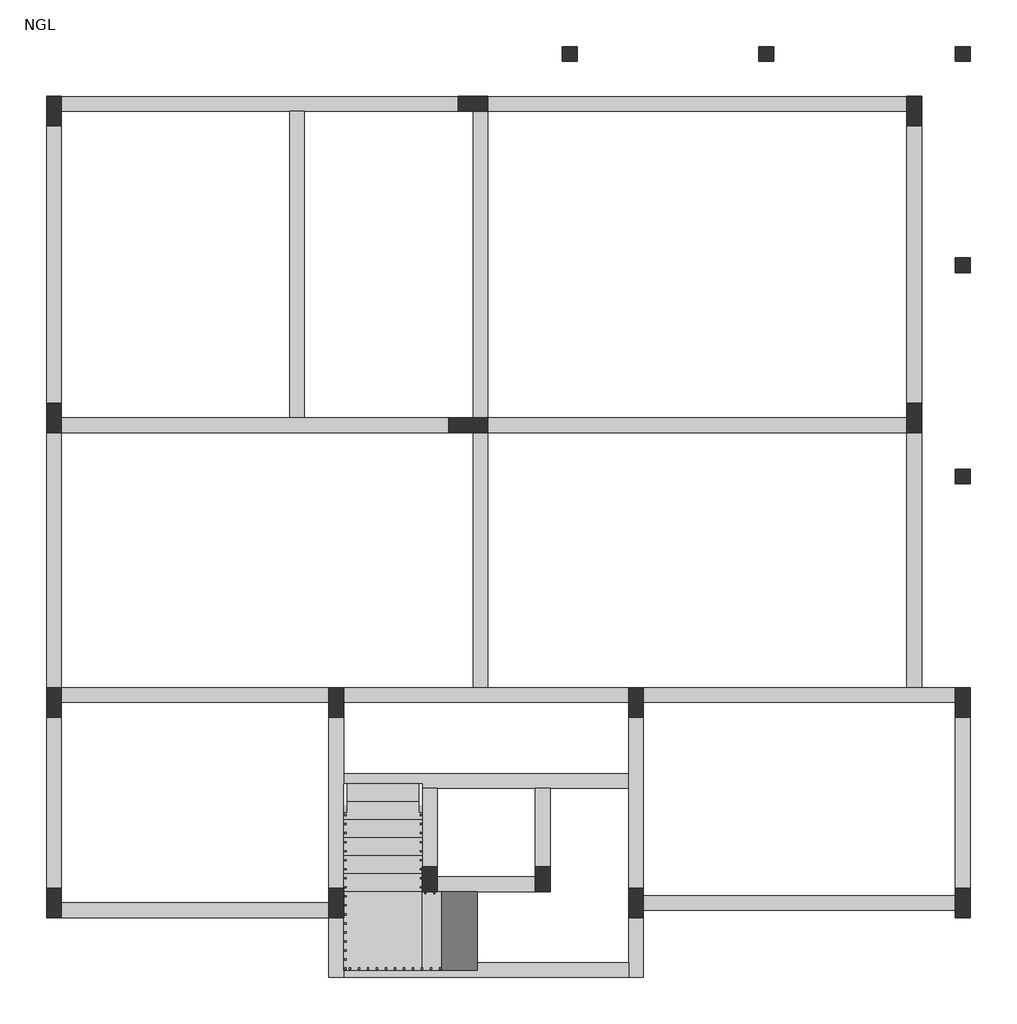
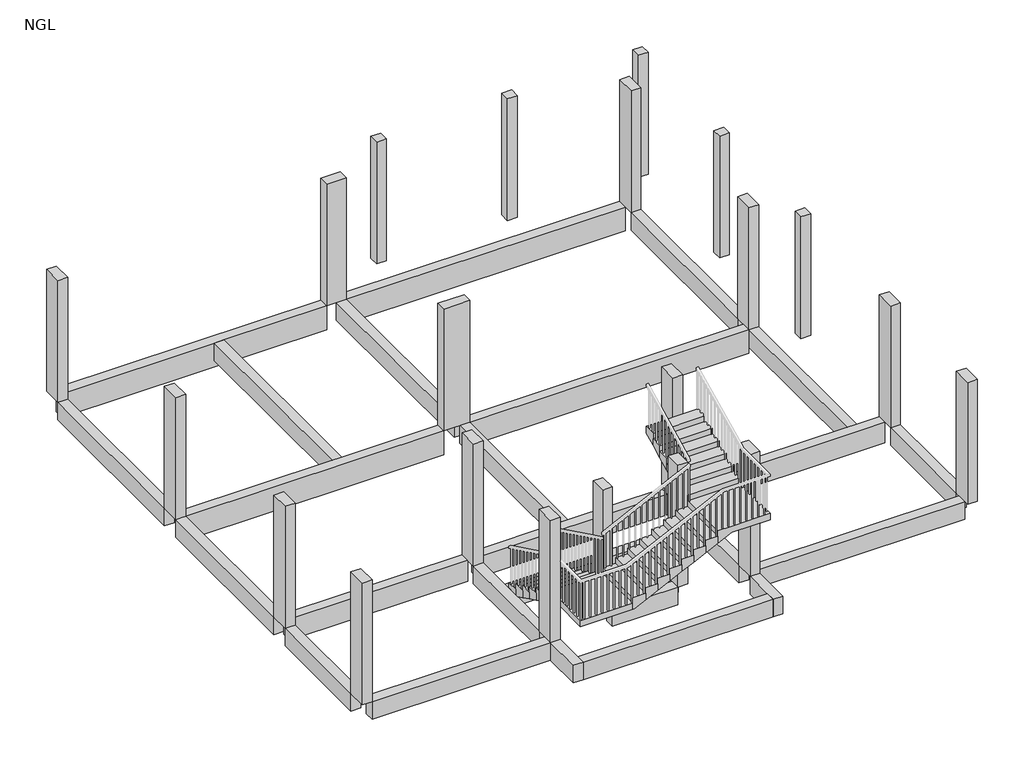
# One storey, part 1 of 2: 27 beams, 21 columns, 1 stair flight.
"""IFC4 building model written with IfcOpenShell, lengths in millimetres."""

from ifc_helpers import new_model, si_unit, frame, origin, origin_with_axes, place, context, project, spatial, polyline, outline, extrude, faceted_brep, transform, mapped, element, save
from components import concrete_rectangular_column_c_80bd43f1

model = new_model("IFC4")

# Units and contexts
model_context = context("Model", 3, world=origin())
ifc_project = project(units=[si_unit("LENGTHUNIT", "METRE", prefix="MILLI")], contexts=[model_context])

# Site, building, storey
site = spatial("IfcSite", under=ifc_project)
building = spatial("IfcBuilding", under=site)
storey = spatial("IfcBuildingStorey", under=building, Name="NGL", Elevation=0.0)

# Beams
placement = place(None, origin())
element("IfcBeam", 1, ObjectType="Concrete - Rectangular Beam : B1", at=placement, inside=storey, context=model_context, shape_type="Brep", body=[
    faceted_brep([(5662813.1113073, -3585265.1224803, 0.0), (5662813.1113073, -3585493.7224803, 0.0), (5666356.4266467, -3585493.7224803, 0.0), (5666585.0266467, -3585493.7224803, 0.0), (5668972.6206949, -3585493.7224803, 0.0), (5668972.6206949, -3585265.1224803, 0.0), (5662813.1113073, -3585493.7224803, -584.2), (5668972.6206949, -3585493.7224803, -584.2), (5662813.1113073, -3585265.1224803, -584.2), (5668972.6206949, -3585265.1224803, -584.2)], [[[0, 1, 2, 3, 4, 5]], [[1, 6, 7, 4, 3, 2]], [[6, 8, 9, 7]], [[8, 0, 5, 9]], [[1, 0, 8, 6]], [[5, 4, 7, 9]]]),
])
element("IfcBeam", 2, ObjectType="Concrete - Rectangular Beam : B1", at=placement, inside=storey, context=model_context, shape_type="Brep", body=[
    faceted_brep([(5675932.2165246, -3585493.7224803, 0.0), (5675932.2165246, -3585265.1224803, 0.0), (5669429.8206949, -3585265.1224803, 0.0), (5669429.8297535, -3585493.7224803, 0.0), (5675932.2165246, -3585493.7224803, -584.2), (5669429.8206949, -3585493.7224803, -584.2), (5675932.2165246, -3585265.1224803, -584.2), (5669429.8206949, -3585265.1224803, -584.2)], [[[0, 1, 2, 3]], [[4, 0, 3, 5]], [[6, 4, 5, 7]], [[1, 6, 7, 2]], [[1, 0, 4, 6]], [[2, 7, 5, 3]]]),
])
element("IfcBeam", 3, ObjectType="Concrete - Rectangular Beam : B10", at=placement, inside=storey, context=model_context, shape_type="SweptSolid", body=[
    extrude(outline(polyline([(5670395.0165245, -3597217.2875145), (5670166.4165245, -3597217.2875145), (5670166.4165245, -3595998.1287586), (5670395.0165245, -3595998.1287586), (5670395.0165245, -3597217.2875145)])), frame((0.0, 0.0, -431.8), z_axis=(0.0, 0.0, 1.0), x_axis=(1.0, 0.0, 0.0)), (0.0, 0.0, 1.0), 431.8),
])
element("IfcBeam", 4, ObjectType="Concrete - Rectangular Beam : B10", at=placement, inside=storey, context=model_context, shape_type="SweptSolid", body=[
    extrude(outline(polyline([(5668642.4165246, -3597217.2875145), (5668413.8165246, -3597217.2875145), (5668413.8165246, -3595998.1287586), (5668642.4165246, -3595998.1287586), (5668642.4165246, -3597217.2875145)])), frame((0.0, 0.0, -431.8), z_axis=(0.0, 0.0, 1.0), x_axis=(1.0, 0.0, 0.0)), (0.0, 0.0, 1.0), 431.8),
])
element("IfcBeam", 5, ObjectType="Concrete - Rectangular Beam : B11", at=placement, inside=storey, context=model_context, shape_type="SweptSolid", body=[
    extrude(outline(polyline([(5669201.2297535, -3585493.7224803), (5669429.8297535, -3585493.7224803), (5669429.8297535, -3590249.6682909), (5669201.2297535, -3590249.6682909), (5669201.2297535, -3585493.7224803)])), frame((0.0, 0.0, -431.8), z_axis=(0.0, 0.0, 1.0), x_axis=(1.0, 0.0, 0.0)), (0.0, 0.0, 1.0), 431.8),
])
element("IfcBeam", 6, ObjectType="Concrete - Rectangular Beam : B11", at=placement, inside=storey, context=model_context, shape_type="SweptSolid", body=[
    extrude(outline(polyline([(5669201.2297535, -3590478.2682909), (5669429.8297535, -3590478.2682909), (5669429.8297535, -3594436.7630076), (5669201.2297535, -3594436.7630076), (5669201.2297535, -3590478.2682909)])), frame((0.0, 0.0, -431.8), z_axis=(0.0, 0.0, 1.0), x_axis=(1.0, 0.0, 0.0)), (0.0, 0.0, 1.0), 431.8),
])
element("IfcBeam", 7, ObjectType="Concrete - Rectangular Beam : B12", at=placement, inside=storey, context=model_context, shape_type="SweptSolid", body=[
    extrude(outline(polyline([(5675932.2165246, -3585722.3224803), (5676160.8165246, -3585722.3224803), (5676160.8165246, -3590021.0682909), (5675932.2165246, -3590021.0682909), (5675932.2165246, -3585722.3224803)])), frame((0.0, 0.0, -431.8), z_axis=(0.0, 0.0, 1.0), x_axis=(1.0, 0.0, 0.0)), (0.0, 0.0, 1.0), 431.8),
])
element("IfcBeam", 8, ObjectType="Concrete - Rectangular Beam : B12", at=placement, inside=storey, context=model_context, shape_type="SweptSolid", body=[
    extrude(outline(polyline([(5675932.2165246, -3590478.2682909), (5676160.8165246, -3590478.2682909), (5676160.8165246, -3594436.7630076), (5675932.2165246, -3594436.7630076), (5675932.2165246, -3590478.2682909)])), frame((0.0, 0.0, -431.8), z_axis=(0.0, 0.0, 1.0), x_axis=(1.0, 0.0, 0.0)), (0.0, 0.0, 1.0), 431.8),
])
element("IfcBeam", 9, ObjectType="Concrete - Rectangular Beam : B13", at=placement, inside=storey, context=model_context, shape_type="SweptSolid", body=[
    extrude(outline(polyline([(5676681.5650571, -3594893.8523052), (5676910.1650571, -3594893.8523052), (5676910.1650571, -3597545.8975754), (5676681.5650571, -3597545.8975754), (5676681.5650571, -3594893.8523052)])), frame((0.0, 0.0, -431.8), z_axis=(0.0, 0.0, 1.0), x_axis=(1.0, 0.0, 0.0)), (0.0, 0.0, 1.0), 431.8),
])
element("IfcBeam", 10, ObjectType="Concrete - Rectangular Beam : B2", at=placement, inside=storey, context=model_context, shape_type="Brep", body=[
    faceted_brep([(5668820.2206949, -3590478.2682909, 0.0), (5668820.2206949, -3590249.6682909, 0.0), (5666585.0266467, -3590249.6682909, 0.0), (5666356.4266467, -3590249.6682909, 0.0), (5662813.1650571, -3590249.6682909, 0.0), (5662813.1650571, -3590478.2682909, 0.0), (5668820.2206949, -3590478.2682909, -584.2), (5662813.1650571, -3590478.2682909, -584.2), (5668820.2206949, -3590249.6682909, -584.2), (5662813.1650571, -3590249.6682909, -584.2)], [[[0, 1, 2, 3, 4, 5]], [[6, 0, 5, 7]], [[8, 6, 7, 9]], [[1, 8, 9, 4, 3, 2]], [[1, 0, 6, 8]], [[5, 4, 9, 7]]]),
])
element("IfcBeam", 11, ObjectType="Concrete - Rectangular Beam : B2", at=placement, inside=storey, context=model_context, shape_type="Brep", body=[
    faceted_brep([(5675932.2165246, -3590478.2682909, 0.0), (5675932.2165246, -3590249.6682909, 0.0), (5669429.8297535, -3590249.6682909, 0.0), (5669429.8206949, -3590478.2682909, 0.0), (5675932.2165246, -3590478.2682909, -584.2), (5669429.8206949, -3590478.2682909, -584.2), (5675932.2165246, -3590249.6682909, -584.2), (5669429.8206949, -3590249.6682909, -584.2)], [[[0, 1, 2, 3]], [[4, 0, 3, 5]], [[6, 4, 5, 7]], [[1, 6, 7, 2]], [[1, 0, 4, 6]], [[7, 5, 3, 2]]]),
])
element("IfcBeam", 12, ObjectType="Concrete - Rectangular Beam : B3", at=placement, inside=storey, context=model_context, shape_type="SweptSolid", body=[
    extrude(outline(polyline([(5662813.1650571, -3594665.3630076), (5662813.1650571, -3594436.7630076), (5666966.0165246, -3594436.7630076), (5666966.0165246, -3594665.3630076), (5662813.1650571, -3594665.3630076)])), frame((0.0, 0.0, -508.0), z_axis=(0.0, 0.0, 1.0), x_axis=(1.0, 0.0, 0.0)), (0.0, 0.0, 1.0), 508.0),
])
element("IfcBeam", 13, ObjectType="Concrete - Rectangular Beam : B3", at=placement, inside=storey, context=model_context, shape_type="Brep", body=[
    faceted_brep([(5667194.6165246, -3594436.7630076, 0.0), (5667194.6165246, -3594665.3630076, 0.0), (5671614.2165246, -3594665.3630076, 0.0), (5671614.2165246, -3594436.7630076, 0.0), (5669429.8297535, -3594436.7630076, 0.0), (5669201.2297535, -3594436.7630076, 0.0), (5667194.6165246, -3594665.3630076, -508.0), (5671614.2165246, -3594665.3630076, -508.0), (5667194.6165246, -3594436.7630076, -508.0), (5671614.2165246, -3594436.7630076, -508.0)], [[[0, 1, 2, 3, 4, 5]], [[1, 6, 7, 2]], [[6, 8, 9, 7]], [[8, 0, 5, 4, 3, 9]], [[1, 0, 8, 6]], [[3, 2, 7, 9]]]),
])
element("IfcBeam", 14, ObjectType="Concrete - Rectangular Beam : B3", at=placement, inside=storey, context=model_context, shape_type="Brep", body=[
    faceted_brep([(5671842.8165246, -3594436.7630076, 0.0), (5671842.8165246, -3594665.3630076, 0.0), (5676681.5650571, -3594665.3630076, 0.0), (5676681.5650571, -3594436.7630076, 0.0), (5676160.8165246, -3594436.7630076, 0.0), (5675932.2165246, -3594436.7630076, 0.0), (5671842.8165246, -3594665.3630076, -508.0), (5676681.5650571, -3594665.3630076, -508.0), (5671842.8165246, -3594436.7630076, -508.0), (5676681.5650571, -3594436.7630076, -508.0)], [[[0, 1, 2, 3, 4, 5]], [[1, 6, 7, 2]], [[6, 8, 9, 7]], [[8, 0, 5, 4, 3, 9]], [[1, 0, 8, 6]], [[3, 2, 7, 9]]]),
])
element("IfcBeam", 15, ObjectType="Concrete - Rectangular Beam : B4", at=placement, inside=storey, context=model_context, shape_type="Brep", body=[
    faceted_brep([(5667194.5730158, -3595998.1287586, 0.0), (5667194.5730158, -3595769.5287586, 0.0), (5667194.5730158, -3595769.5287586, -431.8), (5667194.5730158, -3595998.1287586, -431.8), (5668413.8165246, -3595998.1287586, 0.0), (5668642.4165246, -3595998.1287586, 0.0), (5670166.4165245, -3595998.1287586, 0.0), (5670395.0165245, -3595998.1287586, 0.0), (5671614.2165246, -3595998.1287586, 0.0), (5671614.2165246, -3595769.5287586, 0.0), (5671614.2165246, -3595769.5287586, -431.8), (5671614.2165246, -3595998.1287586, -431.8), (5670395.0165245, -3595998.1287586, -431.8), (5670166.4165245, -3595998.1287586, -431.8), (5668642.4165246, -3595998.1287586, -431.8), (5668413.8165246, -3595998.1287586, -431.8)], [[[0, 1, 2, 3]], [[1, 0, 4, 5, 6, 7, 8, 9]], [[2, 1, 9, 10]], [[3, 2, 10, 11, 12, 13, 14, 15]], [[0, 3, 15, 14, 13, 12, 11, 8, 7, 6, 5, 4]], [[9, 8, 11, 10]]]),
])
element("IfcBeam", 16, ObjectType="Concrete - Rectangular Beam : B5", at=placement, inside=storey, context=model_context, shape_type="SweptSolid", body=[
    extrude(outline(polyline([(5666966.0165246, -3597772.5970254), (5666966.0165246, -3598001.1970254), (5662813.1113073, -3598001.1970254), (5662813.1113073, -3597772.5970254), (5666966.0165246, -3597772.5970254)])), frame((0.0, 0.0, -431.8), z_axis=(0.0, 0.0, 1.0), x_axis=(1.0, 0.0, 0.0)), (0.0, 0.0, 1.0), 431.8),
])
element("IfcBeam", 17, ObjectType="Concrete - Rectangular Beam : B5", at=placement, inside=storey, context=model_context, shape_type="Brep", body=[
    faceted_brep([(5671842.8165246, -3597660.1975754, 0.0), (5671842.8165246, -3597888.7975754, 0.0), (5676681.5113073, -3597888.7975754, 0.0), (5676681.5650571, -3597660.1975754, 0.0), (5671842.8165246, -3597660.1975754, -431.8), (5676681.5650571, -3597660.1975754, -431.8), (5671842.8165246, -3597888.7975754, -431.8), (5676681.5113073, -3597888.7975754, -431.8)], [[[0, 1, 2, 3]], [[4, 0, 3, 5]], [[6, 4, 5, 7]], [[1, 6, 7, 2]], [[0, 4, 6, 1]], [[2, 7, 5, 3]]]),
])
element("IfcBeam", 18, ObjectType="Concrete - Rectangular Beam : B6", at=placement, inside=storey, context=model_context, shape_type="SweptSolid", body=[
    extrude(outline(polyline([(5668642.4165246, -3597598.3245381), (5668642.4165246, -3597369.7245381), (5670166.4165245, -3597369.7245381), (5670166.4165245, -3597598.3245381), (5668642.4165246, -3597598.3245381)])), frame((0.0, 0.0, -431.8), z_axis=(0.0, 0.0, 1.0), x_axis=(1.0, 0.0, 0.0)), (0.0, 0.0, 1.0), 431.8),
])
element("IfcBeam", 19, ObjectType="Concrete - Rectangular Beam : B7", at=placement, inside=storey, context=model_context, shape_type="SweptSolid", body=[
    extrude(outline(polyline([(5662584.5113073, -3594893.8523052), (5662813.1113073, -3594893.8523052), (5662813.1113073, -3597545.8975754), (5662584.5113073, -3597545.8975754), (5662584.5113073, -3594893.8523052)])), frame((0.0, 0.0, -431.8), z_axis=(0.0, 0.0, 1.0), x_axis=(1.0, 0.0, 0.0)), (0.0, 0.0, 1.0), 431.8),
])
element("IfcBeam", 20, ObjectType="Concrete - Rectangular Beam : B7", at=placement, inside=storey, context=model_context, shape_type="Brep", body=[
    faceted_brep([(5662813.1650571, -3590478.2682909, 0.0), (5662584.5650571, -3590478.2682909, 0.0), (5662584.5650571, -3594436.6523052, 0.0), (5662813.1650571, -3594436.7630076, 0.0), (5662813.1650571, -3590478.2682909, -431.8), (5662813.1650571, -3594436.7630076, -431.8), (5662584.5650571, -3590478.2682909, -431.8), (5662584.5650571, -3594436.6523052, -431.8)], [[[0, 1, 2, 3]], [[4, 0, 3, 5]], [[6, 4, 5, 7]], [[1, 6, 7, 2]], [[0, 4, 6, 1]], [[2, 7, 5, 3]]]),
])
element("IfcBeam", 21, ObjectType="Concrete - Rectangular Beam : B7", at=placement, inside=storey, context=model_context, shape_type="SweptSolid", body=[
    extrude(outline(polyline([(5662584.5650571, -3585722.3289932), (5662813.1650571, -3585722.3289932), (5662813.1650571, -3590021.0682909), (5662584.5650571, -3590021.0682909), (5662584.5650571, -3585722.3289932)])), frame((0.0, 0.0, -431.8), z_axis=(0.0, 0.0, 1.0), x_axis=(1.0, 0.0, 0.0)), (0.0, 0.0, 1.0), 431.8),
])
element("IfcBeam", 22, ObjectType="Concrete - Rectangular Beam : B8", at=placement, inside=storey, context=model_context, shape_type="SweptSolid", body=[
    extrude(outline(polyline([(5666356.4266467, -3585493.7224803), (5666585.0266467, -3585493.7224803), (5666585.0266467, -3590249.6682909), (5666356.4266467, -3590249.6682909), (5666356.4266467, -3585493.7224803)])), frame((0.0, 0.0, -431.8), z_axis=(0.0, 0.0, 1.0), x_axis=(1.0, 0.0, 0.0)), (0.0, 0.0, 1.0), 431.8),
])
element("IfcBeam", 23, ObjectType="Concrete - Rectangular Beam : B9", at=placement, inside=storey, context=model_context, shape_type="Brep", body=[
    faceted_brep([(5667194.6165246, -3594893.8523052, 0.0), (5666966.0165246, -3594893.8523052, 0.0), (5666966.0165246, -3597545.8975754, 0.0), (5667194.6165246, -3597545.8975754, 0.0), (5667194.6165246, -3595998.1287586, 0.0), (5667194.6165246, -3595769.5287586, 0.0), (5666966.0165246, -3594893.8523052, -431.8), (5666966.0165246, -3597545.8975754, -431.8), (5667194.6165246, -3594893.8523052, -431.8), (5667194.6165246, -3595769.5287586, -431.8), (5667194.6165246, -3595998.1287586, -431.8), (5667194.6165246, -3597545.8975754, -431.8)], [[[0, 1, 2, 3, 4, 5]], [[1, 6, 7, 2]], [[6, 8, 9, 10, 11, 7]], [[8, 0, 5, 4, 3, 11, 10, 9]], [[1, 0, 8, 6]], [[3, 2, 7, 11]]]),
])
element("IfcBeam", 24, ObjectType="Concrete - Rectangular Beam : B9", at=placement, inside=storey, context=model_context, shape_type="Brep", body=[
    faceted_brep([(5671842.8165246, -3594893.8523052, 0.0), (5671614.2165246, -3594893.8523052, 0.0), (5671614.2165246, -3595769.5287586, 0.0), (5671614.2165246, -3595998.1287586, 0.0), (5671614.2165246, -3597545.8975754, 0.0), (5671842.8165246, -3597545.8975754, 0.0), (5671614.2165246, -3594893.8523052, -431.8), (5671614.2165246, -3595769.5287586, -431.8), (5671614.2165246, -3595998.1287586, -431.8), (5671614.2165246, -3597545.8975754, -431.8), (5671842.8165246, -3594893.8523052, -431.8), (5671842.8165246, -3597545.8975754, -431.8)], [[[0, 1, 2, 3, 4, 5]], [[1, 6, 7, 8, 9, 4, 3, 2]], [[6, 10, 11, 9, 8, 7]], [[10, 0, 5, 11]], [[1, 0, 10, 6]], [[5, 4, 9, 11]]]),
])
element("IfcBeam", 25, ObjectType="Concrete - Rectangular Beam : B9", at=placement, inside=storey, context=model_context, shape_type="Brep", body=[
    faceted_brep([(5666966.0165246, -3598930.9157548, 0.0), (5667194.6165246, -3598930.9157548, 0.0), (5667194.6165246, -3598702.3157548, 0.0), (5667194.6165246, -3598003.0975754, 0.0), (5666966.0165246, -3598003.0975754, 0.0), (5666966.0165246, -3598930.9157548, -431.8), (5666966.0165246, -3598003.0975754, -431.8), (5667194.6165246, -3598930.9157548, -431.8), (5667194.6165246, -3598003.0975754, -431.8), (5667194.6165246, -3598702.3157548, -431.8)], [[[0, 1, 2, 3, 4]], [[5, 0, 4, 6]], [[7, 5, 6, 8, 9]], [[1, 7, 9, 8, 3, 2]], [[4, 3, 8, 6]], [[1, 0, 5, 7]]]),
])
element("IfcBeam", 26, ObjectType="Concrete - Rectangular Beam : B9", at=placement, inside=storey, context=model_context, shape_type="Brep", body=[
    faceted_brep([(5671614.2165246, -3598930.9157548, 0.0), (5671842.8165246, -3598930.9157548, 0.0), (5671842.8165246, -3598003.0975754, 0.0), (5671614.2165246, -3598003.0975754, 0.0), (5671614.2165246, -3598702.3157548, 0.0), (5671614.2165246, -3598930.9157548, -431.8), (5671614.2165246, -3598003.0975754, -431.8), (5671614.2165246, -3598702.3157548, -431.8), (5671842.8165246, -3598930.9157548, -431.8), (5671842.8165246, -3598003.0975754, -431.8)], [[[0, 1, 2, 3, 4]], [[5, 0, 4, 3, 6, 7]], [[8, 5, 7, 6, 9]], [[1, 8, 9, 2]], [[3, 2, 9, 6]], [[1, 0, 5, 8]]]),
])
element("IfcBeam", 27, ObjectType="Concrete - Rectangular Beam : B9", at=placement, inside=storey, context=model_context, shape_type="SweptSolid", body=[
    extrude(outline(polyline([(5667194.6165246, -3598930.9157548), (5667194.6165246, -3598702.3157548), (5671614.2165246, -3598702.3157548), (5671614.2165246, -3598930.9157548), (5667194.6165246, -3598930.9157548)])), frame((0.0, 0.0, -431.8), z_axis=(0.0, 0.0, 1.0), x_axis=(1.0, 0.0, 0.0)), (0.0, 0.0, 1.0), 431.8),
])

# Columns
concrete_rectangular_column_c_shape = concrete_rectangular_column_c_80bd43f1(model_context)
element("IfcColumn", 28, ObjectType="Concrete-Rectangular-Column : C", at=placement, inside=storey, context=model_context, shape_type="MappedRepresentation", body=[
    mapped(concrete_rectangular_column_c_shape, transform((5670699.8650571, -3584604.6060698, 0.0), x_axis=(1.0, 0.0, 0.0), y_axis=(0.0, 1.0, 0.0), z_axis=(0.0, 0.0, 1.0))),
])
element("IfcColumn", 29, ObjectType="Concrete-Rectangular-Column : C", at=placement, inside=storey, context=model_context, shape_type="MappedRepresentation", body=[
    mapped(concrete_rectangular_column_c_shape, transform((5673747.8650571, -3584604.6060698, 0.0), x_axis=(1.0, 0.0, 0.0), y_axis=(0.0, 1.0, 0.0), z_axis=(0.0, 0.0, 1.0))),
])
element("IfcColumn", 30, ObjectType="Concrete-Rectangular-Column : C", at=placement, inside=storey, context=model_context, shape_type="MappedRepresentation", body=[
    mapped(concrete_rectangular_column_c_shape, transform((5676795.8650571, -3584604.6060698, 0.0), x_axis=(1.0, 0.0, 0.0), y_axis=(0.0, 1.0, 0.0), z_axis=(0.0, 0.0, 1.0))),
])
element("IfcColumn", 31, ObjectType="Concrete-Rectangular-Column : C", at=placement, inside=storey, context=model_context, shape_type="MappedRepresentation", body=[
    mapped(concrete_rectangular_column_c_shape, transform((5676795.8650571, -3587881.949152, 0.0), x_axis=(1.0, 0.0, 0.0), y_axis=(0.0, 1.0, 0.0), z_axis=(0.0, 0.0, 1.0))),
])
element("IfcColumn", 32, ObjectType="Concrete-Rectangular-Column : C", at=placement, inside=storey, context=model_context, shape_type="MappedRepresentation", body=[
    mapped(concrete_rectangular_column_c_shape, transform((5676795.8650571, -3591159.3007286, 0.0), x_axis=(1.0, 0.0, 0.0), y_axis=(0.0, 1.0, 0.0), z_axis=(0.0, 0.0, 1.0))),
])
element("IfcColumn", 33, ObjectType="Concrete-Rectangular-Column : C1", at=placement, inside=storey, context=model_context, shape_type="SweptSolid", body=[
    extrude(outline(polyline([(5662813.1113073, -3585265.1289932), (5662813.1113073, -3585722.3289932), (5662584.5113073, -3585722.3289932), (5662584.5113073, -3585265.1289932), (5662813.1113073, -3585265.1289932)])), origin_with_axes(), (0.0, 0.0, 1.0), 3000.0),
])
element("IfcColumn", 34, ObjectType="Concrete-Rectangular-Column : C1", at=placement, inside=storey, context=model_context, shape_type="SweptSolid", body=[
    extrude(outline(polyline([(5676160.8165246, -3585265.1224803), (5676160.8165246, -3585722.3224803), (5675932.2165246, -3585722.3224803), (5675932.2165246, -3585265.1224803), (5676160.8165246, -3585265.1224803)])), origin_with_axes(), (0.0, 0.0, 1.0), 3000.0),
])
element("IfcColumn", 35, ObjectType="Concrete-Rectangular-Column : C1", at=placement, inside=storey, context=model_context, shape_type="SweptSolid", body=[
    extrude(outline(polyline([(5662813.1113073, -3597545.8975754), (5662813.1113073, -3598003.0975754), (5662584.5113073, -3598003.0975754), (5662584.5113073, -3597545.8975754), (5662813.1113073, -3597545.8975754)])), origin_with_axes(), (0.0, 0.0, 1.0), 3000.0),
])
element("IfcColumn", 36, ObjectType="Concrete-Rectangular-Column : C1", at=placement, inside=storey, context=model_context, shape_type="SweptSolid", body=[
    extrude(outline(polyline([(5676910.1113073, -3597545.8975754), (5676910.1113073, -3598003.0975754), (5676681.5113073, -3598003.0975754), (5676681.5113073, -3597545.8975754), (5676910.1113073, -3597545.8975754)])), origin_with_axes(), (0.0, 0.0, 1.0), 3000.0),
])
element("IfcColumn", 37, ObjectType="Concrete-Rectangular-Column : C2", at=placement, inside=storey, context=model_context, shape_type="SweptSolid", body=[
    extrude(outline(polyline([(5668972.6206949, -3585265.1224803), (5669429.8206949, -3585265.1224803), (5669429.8206949, -3585493.7224803), (5668972.6206949, -3585493.7224803), (5668972.6206949, -3585265.1224803)])), origin_with_axes(), (0.0, 0.0, 1.0), 3000.0),
])
element("IfcColumn", 38, ObjectType="Concrete-Rectangular-Column : C2", at=placement, inside=storey, context=model_context, shape_type="SweptSolid", body=[
    extrude(outline(polyline([(5676160.8165246, -3590021.0682909), (5676160.8165246, -3590478.2682909), (5675932.2165246, -3590478.2682909), (5675932.2165246, -3590021.0682909), (5676160.8165246, -3590021.0682909)])), origin_with_axes(), (0.0, 0.0, 1.0), 3000.0),
])
element("IfcColumn", 39, ObjectType="Concrete-Rectangular-Column : C2", at=placement, inside=storey, context=model_context, shape_type="SweptSolid", body=[
    extrude(outline(polyline([(5662813.1650571, -3590021.0682909), (5662813.1650571, -3590478.2682909), (5662584.5650571, -3590478.2682909), (5662584.5650571, -3590021.0682909), (5662813.1650571, -3590021.0682909)])), origin_with_axes(), (0.0, 0.0, 1.0), 3000.0),
])
element("IfcColumn", 40, ObjectType="Concrete-Rectangular-Column : C2", at=placement, inside=storey, context=model_context, shape_type="SweptSolid", body=[
    extrude(outline(polyline([(5662813.1650571, -3594436.6523052), (5662813.1650571, -3594893.8523052), (5662584.5650571, -3594893.8523052), (5662584.5650571, -3594436.6523052), (5662813.1650571, -3594436.6523052)])), origin_with_axes(), (0.0, 0.0, 1.0), 3000.0),
])
element("IfcColumn", 41, ObjectType="Concrete-Rectangular-Column : C2", at=placement, inside=storey, context=model_context, shape_type="SweptSolid", body=[
    extrude(outline(polyline([(5667194.6165246, -3594436.6523052), (5667194.6165246, -3594893.8523052), (5666966.0165246, -3594893.8523052), (5666966.0165246, -3594436.6523052), (5667194.6165246, -3594436.6523052)])), origin_with_axes(), (0.0, 0.0, 1.0), 3000.0),
])
element("IfcColumn", 42, ObjectType="Concrete-Rectangular-Column : C2", at=placement, inside=storey, context=model_context, shape_type="SweptSolid", body=[
    extrude(outline(polyline([(5671842.8165246, -3594436.6523052), (5671842.8165246, -3594893.8523052), (5671614.2165246, -3594893.8523052), (5671614.2165246, -3594436.6523052), (5671842.8165246, -3594436.6523052)])), origin_with_axes(), (0.0, 0.0, 1.0), 3000.0),
])
element("IfcColumn", 43, ObjectType="Concrete-Rectangular-Column : C2", at=placement, inside=storey, context=model_context, shape_type="SweptSolid", body=[
    extrude(outline(polyline([(5676910.1650571, -3594436.6523052), (5676910.1650571, -3594893.8523052), (5676681.5650571, -3594893.8523052), (5676681.5650571, -3594436.6523052), (5676910.1650571, -3594436.6523052)])), origin_with_axes(), (0.0, 0.0, 1.0), 3000.0),
])
element("IfcColumn", 44, ObjectType="Concrete-Rectangular-Column : C2", at=placement, inside=storey, context=model_context, shape_type="SweptSolid", body=[
    extrude(outline(polyline([(5671842.8165246, -3597545.8975754), (5671842.8165246, -3598003.0975754), (5671614.2165246, -3598003.0975754), (5671614.2165246, -3597545.8975754), (5671842.8165246, -3597545.8975754)])), origin_with_axes(), (0.0, 0.0, 1.0), 3000.0),
])
element("IfcColumn", 45, ObjectType="Concrete-Rectangular-Column : C2", at=placement, inside=storey, context=model_context, shape_type="SweptSolid", body=[
    extrude(outline(polyline([(5667194.6165246, -3597545.8975754), (5667194.6165246, -3598003.0975754), (5666966.0165246, -3598003.0975754), (5666966.0165246, -3597545.8975754), (5667194.6165246, -3597545.8975754)])), origin_with_axes(), (0.0, 0.0, 1.0), 3000.0),
])
element("IfcColumn", 46, ObjectType="Concrete-Rectangular-Column : C3", at=placement, inside=storey, context=model_context, shape_type="SweptSolid", body=[
    extrude(outline(polyline([(5668820.2206949, -3590249.6682909), (5669429.8206949, -3590249.6682909), (5669429.8206949, -3590478.2682909), (5668820.2206949, -3590478.2682909), (5668820.2206949, -3590249.6682909)])), origin_with_axes(), (0.0, 0.0, 1.0), 3000.0),
])
element("IfcColumn", 47, ObjectType="Concrete-Rectangular-Column : C4", at=placement, inside=storey, context=model_context, shape_type="SweptSolid", body=[
    extrude(outline(polyline([(5668642.4165246, -3597217.2875145), (5668642.4165246, -3597598.2875145), (5668413.8165246, -3597598.2875145), (5668413.8165246, -3597217.2875145), (5668642.4165246, -3597217.2875145)])), origin_with_axes(), (0.0, 0.0, 1.0), 3000.0),
])
element("IfcColumn", 48, ObjectType="Concrete-Rectangular-Column : C4", at=placement, inside=storey, context=model_context, shape_type="SweptSolid", body=[
    extrude(outline(polyline([(5670395.0165245, -3597217.2875145), (5670395.0165245, -3597598.2875145), (5670166.4165245, -3597598.2875145), (5670166.4165245, -3597217.2875145), (5670395.0165245, -3597217.2875145)])), origin_with_axes(), (0.0, 0.0, 1.0), 3000.0),
])

# Stair flight
element("IfcStairFlight", 49, ObjectType="25 mm Nosing", at=placement, inside=storey, context=model_context, shape_type="Brep", body=[
    faceted_brep([(5668413.8165246, -3596201.8258983, 136.3636364), (5668413.8165246, -3595922.4258983, 136.3636364), (5667194.6165246, -3595922.4258983, 136.3636364), (5667194.6165246, -3596201.8258983, 136.3636364), (5668413.8165246, -3596201.8258983, 0.0), (5668413.8165246, -3595922.4258983, 0.0), (5667194.6165246, -3595922.4258983, 0.0), (5667194.6165246, -3596201.8258983, 0.0), (5668413.8165246, -3596481.2258983, 272.7272727), (5668413.8165246, -3596201.8258983, 272.7272727), (5667194.6165246, -3596201.8258983, 272.7272727), (5667194.6165246, -3596481.2258983, 272.7272727), (5668413.8165246, -3596481.2258983, 105.8155238), (5668413.8165246, -3596264.4169444, 0.0), (5667194.6165246, -3596264.4169444, 0.0), (5667194.6165246, -3596481.2258983, 105.8155238), (5668413.8165246, -3596760.6258983, 409.0909091), (5668413.8165246, -3596481.2258983, 409.0909091), (5667194.6165246, -3596481.2258983, 409.0909091), (5667194.6165246, -3596760.6258983, 409.0909091), (5668413.8165246, -3596760.6258983, 242.1791602), (5667194.6165246, -3596760.6258983, 242.1791602), (5668413.8165246, -3597040.0258983, 545.4545455), (5668413.8165246, -3596760.6258983, 545.4545455), (5667194.6165246, -3596760.6258983, 545.4545455), (5667194.6165246, -3597040.0258983, 545.4545455), (5668413.8165246, -3597040.0258983, 378.5427965), (5667194.6165246, -3597040.0258983, 378.5427965), (5668413.8165246, -3597319.4258983, 681.8181818), (5668413.8165246, -3597040.0258983, 681.8181818), (5667194.6165246, -3597040.0258983, 681.8181818), (5667194.6165246, -3597319.4258983, 681.8181818), (5668413.8165246, -3597319.4258983, 514.9064329), (5667194.6165246, -3597319.4258983, 514.9064329), (5668413.8165246, -3597598.8258983, 818.1818182), (5668413.8165246, -3597319.4258983, 818.1818182), (5667194.6165246, -3597319.4258983, 818.1818182), (5667194.6165246, -3597598.8258983, 818.1818182), (5668413.8165246, -3597598.8258983, 804.5454545), (5668413.8165246, -3597912.8769444, 804.5454545), (5667194.6165246, -3597598.8258983, 651.2700693), (5668413.8165246, -3597598.8258983, 954.5454545), (5667194.6165246, -3597598.8258983, 954.5454545), (5667194.6165246, -3597912.8769444, 954.5454545), (5667194.6165246, -3598818.0258983, 954.5454545), (5668413.8165246, -3598818.0258983, 954.5454545), (5667194.6165246, -3597912.8769444, 804.5454545), (5667194.6165246, -3598818.0258983, 804.5454545), (5668413.8165246, -3597598.8258983, 1090.9090909), (5668413.8165246, -3598818.0258983, 1090.9090909), (5668448.0675875, -3598818.0258983, 1090.9090909), (5668718.5627748, -3598818.0258983, 1090.9090909), (5668718.5627748, -3597598.8258983, 1090.9090909), (5668448.0675875, -3597598.8258983, 1090.9090909), (5668718.5627748, -3597598.8258983, 934.8704856), (5668448.0675875, -3597598.8258983, 804.5454545), (5668413.8165246, -3598818.0258983, 804.5454545), (5668448.0675875, -3598818.0258983, 804.5454545), (5668718.5627748, -3598818.0258983, 934.8704856), (5668997.9627748, -3597598.8258983, 1227.2727273), (5668718.5627748, -3597598.8258983, 1227.2727273), (5668718.5627748, -3598818.0258983, 1227.2727273), (5668997.9627748, -3598818.0258983, 1227.2727273), (5668997.9627748, -3597598.8258983, 1069.4858702), (5668997.9627748, -3598818.0258983, 1069.4858702), (5669277.3627748, -3597598.8258983, 1363.6363636), (5668997.9627748, -3597598.8258983, 1363.6363636), (5668997.9627748, -3598818.0258983, 1363.6363636), (5669277.3627748, -3598818.0258983, 1363.6363636), (5669277.3627748, -3597598.8258983, 1204.1012548), (5669277.3627748, -3598818.0258983, 1204.1012548), (5669556.7627748, -3597598.8258983, 1500.0), (5669277.3627748, -3597598.8258983, 1500.0), (5669277.3627748, -3598818.0258983, 1500.0), (5669556.7627748, -3598818.0258983, 1500.0), (5669556.7627748, -3597598.8258983, 1338.7166394), (5669556.7627748, -3598818.0258983, 1338.7166394), (5669836.1627748, -3597598.8258983, 1636.3636364), (5669556.7627748, -3597598.8258983, 1636.3636364), (5669556.7627748, -3598818.0258983, 1636.3636364), (5669836.1627748, -3598818.0258983, 1636.3636364), (5669836.1627748, -3597598.8258983, 1473.3320241), (5669836.1627748, -3598818.0258983, 1473.3320241), (5670115.5627748, -3597598.8258983, 1772.7272727), (5669836.1627748, -3597598.8258983, 1772.7272727), (5669836.1627748, -3598818.0258983, 1772.7272727), (5670115.5627748, -3598818.0258983, 1772.7272727), (5670115.5627748, -3597598.8258983, 1607.9474087), (5670115.5627748, -3598818.0258983, 1607.9474087), (5670395.0165245, -3597598.8258983, 1909.0909091), (5670115.5627748, -3597598.8258983, 1909.0909091), (5670115.5627748, -3598818.0258983, 1909.0909091), (5670395.0165245, -3598818.0258983, 1909.0909091), (5670395.0165245, -3597598.8258983, 1895.4545455), (5670712.2961589, -3597598.8258983, 1895.4545455), (5670395.0165246, -3598818.0258983, 1742.58869), (5670395.0165245, -3597598.8258983, 2045.4545455), (5670395.0165245, -3598818.0258983, 2045.4545455), (5670712.2961589, -3598818.0258983, 2045.4545455), (5671614.2165246, -3598818.0258983, 2045.4545455), (5671614.2165246, -3597598.8258983, 2045.4545455), (5670712.2961589, -3598818.0258983, 1895.4545455), (5671614.2165246, -3598818.0258983, 1895.4545455), (5670395.0165245, -3597598.8258983, 2181.8181818), (5671614.2165246, -3597598.8258983, 2181.8181818), (5671614.2165246, -3597564.1748522, 2181.8181818), (5671614.2165246, -3597319.4258983, 2181.8181818), (5670395.0165245, -3597319.4258983, 2181.8181818), (5670395.0165246, -3597564.1748522, 2181.8181818), (5670395.0165245, -3597319.4258983, 2014.9064329), (5670395.0165245, -3597564.1748522, 1895.4545455), (5671614.2165246, -3597598.8258983, 1895.4545455), (5671614.2165246, -3597564.1748522, 1895.4545455), (5671614.2165246, -3597319.4258983, 2014.9064329), (5670395.0165245, -3597040.0258983, 2318.1818182), (5670395.0165245, -3597319.4258983, 2318.1818182), (5671614.2165246, -3597319.4258983, 2318.1818182), (5671614.2165246, -3597040.0258983, 2318.1818182), (5670395.0165245, -3597040.0258983, 2151.2700693), (5671614.2165246, -3597040.0258983, 2151.2700693), (5670395.0165245, -3596760.6258983, 2454.5454545), (5670395.0165245, -3597040.0258983, 2454.5454545), (5671614.2165246, -3597040.0258983, 2454.5454545), (5671614.2165246, -3596760.6258983, 2454.5454545), (5670395.0165245, -3596760.6258983, 2287.6337056), (5671614.2165246, -3596760.6258983, 2287.6337056), (5670395.0165245, -3596481.2258983, 2590.9090909), (5670395.0165245, -3596760.6258983, 2590.9090909), (5671614.2165246, -3596760.6258983, 2590.9090909), (5671614.2165246, -3596481.2258983, 2590.9090909), (5670395.0165245, -3596481.2258983, 2423.997342), (5671614.2165246, -3596481.2258983, 2423.997342), (5670395.0165245, -3596201.8258983, 2727.2727273), (5670395.0165245, -3596481.2258983, 2727.2727273), (5671614.2165246, -3596481.2258983, 2727.2727273), (5671614.2165246, -3596201.8258983, 2727.2727273), (5670395.0165245, -3596201.8258983, 2560.3609784), (5671614.2165246, -3596201.8258983, 2560.3609784), (5670395.0165245, -3595922.4258983, 2696.7246147), (5671614.2165246, -3595922.4258983, 2696.7246147), (5670395.0165245, -3595922.4258983, 2863.6363636), (5670395.0165245, -3596201.8258983, 2863.6363636), (5671614.2165246, -3596201.8258983, 2863.6363636), (5671614.2165246, -3595922.4258983, 2863.6363636)], [[[0, 1, 2, 3]], [[1, 0, 4, 5]], [[2, 1, 5, 6]], [[3, 2, 6, 7]], [[8, 9, 10, 11]], [[4, 0, 9, 8, 12, 13]], [[0, 3, 10, 9]], [[3, 7, 14, 15, 11, 10]], [[16, 17, 18, 19]], [[17, 16, 20, 12, 8]], [[8, 11, 18, 17]], [[19, 18, 11, 15, 21]], [[22, 23, 24, 25]], [[23, 22, 26, 20, 16]], [[16, 19, 24, 23]], [[25, 24, 19, 21, 27]], [[28, 29, 30, 31]], [[29, 28, 32, 26, 22]], [[22, 25, 30, 29]], [[31, 30, 25, 27, 33]], [[34, 35, 36, 37]], [[35, 34, 38, 39, 32, 28]], [[28, 31, 36, 35]], [[37, 36, 31, 33, 40]], [[41, 42, 43, 44, 45]], [[34, 37, 42, 41]], [[42, 37, 40, 46, 47, 44, 43]], [[48, 49, 50, 51, 52, 53]], [[34, 41, 48, 53, 52, 54, 55, 38]], [[41, 45, 49, 48]], [[49, 45, 56, 57, 58, 51, 50]], [[59, 60, 61, 62]], [[60, 59, 63, 54, 52]], [[52, 51, 61, 60]], [[62, 61, 51, 58, 64]], [[65, 66, 67, 68]], [[66, 65, 69, 63, 59]], [[59, 62, 67, 66]], [[68, 67, 62, 64, 70]], [[71, 72, 73, 74]], [[72, 71, 75, 69, 65]], [[65, 68, 73, 72]], [[74, 73, 68, 70, 76]], [[77, 78, 79, 80]], [[78, 77, 81, 75, 71]], [[71, 74, 79, 78]], [[80, 79, 74, 76, 82]], [[83, 84, 85, 86]], [[84, 83, 87, 81, 77]], [[77, 80, 85, 84]], [[86, 85, 80, 82, 88]], [[89, 90, 91, 92]], [[90, 89, 93, 94, 87, 83]], [[83, 86, 91, 90]], [[92, 91, 86, 88, 95]], [[96, 97, 98, 99, 100]], [[89, 92, 97, 96]], [[97, 92, 95, 101, 102, 99, 98]], [[103, 104, 105, 106, 107, 108]], [[89, 96, 103, 108, 107, 109, 110, 93]], [[96, 100, 104, 103]], [[104, 100, 111, 112, 113, 106, 105]], [[114, 115, 116, 117]], [[115, 114, 118, 109, 107]], [[107, 106, 116, 115]], [[117, 116, 106, 113, 119]], [[120, 121, 122, 123]], [[121, 120, 124, 118, 114]], [[114, 117, 122, 121]], [[123, 122, 117, 119, 125]], [[126, 127, 128, 129]], [[127, 126, 130, 124, 120]], [[120, 123, 128, 127]], [[129, 128, 123, 125, 131]], [[132, 133, 134, 135]], [[133, 132, 136, 130, 126]], [[126, 129, 134, 133]], [[135, 134, 129, 131, 137]], [[5, 4, 13, 14, 7, 6]], [[32, 39, 46, 40, 33, 27, 21, 15, 14, 13, 12, 20, 26]], [[46, 39, 38, 55, 57, 56, 47]], [[57, 55, 54, 63, 69, 75, 81, 87, 94, 101, 95, 88, 82, 76, 70, 64, 58]], [[101, 94, 93, 110, 112, 111, 102]], [[112, 110, 109, 118, 124, 130, 136, 138, 139, 137, 131, 125, 119, 113]], [[45, 44, 47, 56]], [[100, 99, 102, 111]], [[140, 141, 142, 143]], [[141, 140, 138, 136, 132]], [[132, 135, 142, 141]], [[143, 142, 135, 137, 139]], [[140, 143, 139, 138]]]),
])

save(model, "model.ifc")

# Revit data of these elements
# Type "Concrete - Rectangular Beam : B1"
#   Keynote = "E"
#   Length [instance default] = 1524 mm
#   b = 228.6 mm
#   h = 584.2 mm
#   Structural Material [instance default] = Concrete - Cast-in-Place Concrete
#   Assembly Code = ""
# Type "Concrete - Rectangular Beam : B10"
#   Keynote = "E"
#   Length [instance default] = 1524 mm
#   b = 228.6 mm
#   h = 431.8 mm
#   Structural Material [instance default] = Concrete - Cast-in-Place Concrete
#   Assembly Code = ""
# Type "Concrete - Rectangular Beam : B11"
#   Keynote = "E"
#   Length [instance default] = 1524 mm
#   b = 228.6 mm
#   h = 431.8 mm
#   Structural Material [instance default] = Concrete - Cast-in-Place Concrete
#   Assembly Code = ""
# Type "Concrete - Rectangular Beam : B12"
#   Keynote = "E"
#   Length [instance default] = 1524 mm
#   b = 228.6 mm
#   h = 431.8 mm
#   Structural Material [instance default] = Concrete - Cast-in-Place Concrete
#   Assembly Code = ""
# Type "Concrete - Rectangular Beam : B13"
#   Keynote = "E"
#   Length [instance default] = 1524 mm
#   b = 228.6 mm
#   h = 431.8 mm
#   Structural Material [instance default] = Concrete - Cast-in-Place Concrete
#   Assembly Code = ""
# Type "Concrete - Rectangular Beam : B2"
#   Keynote = "E"
#   Length [instance default] = 1524 mm
#   b = 228.6 mm
#   h = 584.2 mm
#   Structural Material [instance default] = Concrete - Cast-in-Place Concrete
#   Assembly Code = ""
# Type "Concrete - Rectangular Beam : B3"
#   Keynote = "E"
#   Length [instance default] = 1524 mm
#   b = 228.6 mm
#   h = 508 mm
#   Structural Material [instance default] = Concrete - Cast-in-Place Concrete
#   Assembly Code = ""
# Type "Concrete - Rectangular Beam : B4"
#   Keynote = "E"
#   Length [instance default] = 1524 mm
#   b = 228.6 mm
#   h = 431.8 mm
#   Structural Material [instance default] = Concrete - Cast-in-Place Concrete
#   Assembly Code = ""
# Type "Concrete - Rectangular Beam : B5"
#   Keynote = "E"
#   Length [instance default] = 1524 mm
#   b = 228.6 mm
#   h = 431.8 mm
#   Structural Material [instance default] = Concrete - Cast-in-Place Concrete
#   Assembly Code = ""
# Type "Concrete - Rectangular Beam : B6"
#   Keynote = "E"
#   Length [instance default] = 1524 mm
#   b = 228.6 mm
#   h = 431.8 mm
#   Structural Material [instance default] = Concrete - Cast-in-Place Concrete
#   Assembly Code = ""
# Type "Concrete - Rectangular Beam : B7"
#   Keynote = "E"
#   Length [instance default] = 1524 mm
#   b = 228.6 mm
#   h = 431.8 mm
#   Structural Material [instance default] = Concrete - Cast-in-Place Concrete
#   Assembly Code = ""
# Type "Concrete - Rectangular Beam : B8"
#   Keynote = "E"
#   Length [instance default] = 1524 mm
#   b = 228.6 mm
#   h = 431.8 mm
#   Structural Material [instance default] = Concrete - Cast-in-Place Concrete
#   Assembly Code = ""
# Type "Concrete - Rectangular Beam : B9"
#   Keynote = "E"
#   Length [instance default] = 1524 mm
#   b = 228.6 mm
#   h = 431.8 mm
#   Structural Material [instance default] = Concrete - Cast-in-Place Concrete
#   Assembly Code = ""
# Type "Concrete-Rectangular-Column : C"
#   b = 228.6 mm
#   h = 228.6 mm
#   Structural Material [instance default] = Concrete, Cast-in-Place gray
# Type "Concrete-Rectangular-Column : C1"
#   b = 228.6 mm
#   h = 457.2 mm
#   Structural Material [instance default] = Concrete, Cast-in-Place gray
# Type "Concrete-Rectangular-Column : C2"
#   b = 228.6 mm
#   h = 457.2 mm
#   Structural Material [instance default] = Concrete, Cast-in-Place gray
# Type "Concrete-Rectangular-Column : C3"
#   b = 228.6 mm
#   h = 609.6 mm
#   Structural Material [instance default] = Concrete, Cast-in-Place gray
# Type "Concrete-Rectangular-Column : C4"
#   b = 228.6 mm
#   h = 381 mm
#   Structural Material [instance default] = Concrete, Cast-in-Place gray
# Elements 1, 2 (IfcBeam, "Concrete - Rectangular Beam : B1")
#   Structural Material = Concrete - Cast-in-Place Concrete
#   Phase Created = New Construction
#   Materials on its faces: "Concrete - Cast-in-Place Concrete"
# Elements 3, 4 (IfcBeam, "Concrete - Rectangular Beam : B10")
#   Length = 1524 mm
#   Structural Material = Concrete - Cast-in-Place Concrete
#   Phase Created = New Construction
#   Materials on its faces: "Concrete - Cast-in-Place Concrete"
# Elements 5, 6 (IfcBeam, "Concrete - Rectangular Beam : B11")
#   Structural Material = Concrete - Cast-in-Place Concrete
#   Phase Created = New Construction
#   Materials on its faces: "Concrete - Cast-in-Place Concrete"
# Elements 7, 8 (IfcBeam, "Concrete - Rectangular Beam : B12")
#   Structural Material = Concrete - Cast-in-Place Concrete
#   Phase Created = New Construction
#   Materials on its faces: "Concrete - Cast-in-Place Concrete"
# Element 9 (IfcBeam, "Concrete - Rectangular Beam : B13")
#   Structural Material = Concrete - Cast-in-Place Concrete
#   Phase Created = New Construction
#   Materials on its faces: "Concrete - Cast-in-Place Concrete"
# Elements 10, 11 (IfcBeam, "Concrete - Rectangular Beam : B2")
#   Structural Material = Concrete - Cast-in-Place Concrete
#   Phase Created = New Construction
#   Materials on its faces: "Concrete - Cast-in-Place Concrete"
# Elements 12, 13, 14 (IfcBeam, "Concrete - Rectangular Beam : B3")
#   Structural Material = Concrete - Cast-in-Place Concrete
#   Phase Created = New Construction
#   Materials on its faces: "Concrete - Cast-in-Place Concrete"
# Element 15 (IfcBeam, "Concrete - Rectangular Beam : B4")
#   Structural Material = Concrete - Cast-in-Place Concrete
#   Phase Created = New Construction
#   Materials on its faces: "Concrete - Cast-in-Place Concrete"
# Elements 16, 17 (IfcBeam, "Concrete - Rectangular Beam : B5")
#   Structural Material = Concrete - Cast-in-Place Concrete
#   Phase Created = New Construction
#   Materials on its faces: "Concrete - Cast-in-Place Concrete"
# Element 18 (IfcBeam, "Concrete - Rectangular Beam : B6")
#   Structural Material = Concrete - Cast-in-Place Concrete
#   Phase Created = New Construction
#   Materials on its faces: "Concrete - Cast-in-Place Concrete"
# Elements 19, 20, 21 (IfcBeam, "Concrete - Rectangular Beam : B7")
#   Structural Material = Concrete - Cast-in-Place Concrete
#   Phase Created = New Construction
#   Materials on its faces: "Concrete - Cast-in-Place Concrete"
# Element 22 (IfcBeam, "Concrete - Rectangular Beam : B8")
#   Structural Material = Concrete - Cast-in-Place Concrete
#   Phase Created = New Construction
#   Materials on its faces: "Concrete - Cast-in-Place Concrete"
# Elements 23, 24, 25, 26, 27 (IfcBeam, "Concrete - Rectangular Beam : B9")
#   Structural Material = Concrete - Cast-in-Place Concrete
#   Phase Created = New Construction
#   Materials on its faces: "Concrete - Cast-in-Place Concrete"
# Elements 28, 29, 30, 31, 32 (IfcColumn, "Concrete-Rectangular-Column : C")
#   Structural Material = Concrete, Cast-in-Place gray
#   Phase Created = New Construction
#   Materials on its faces: "Concrete, Cast-in-Place gray"
# Elements 33, 34, 35, 36 (IfcColumn, "Concrete-Rectangular-Column : C1")
#   Structural Material = Concrete, Cast-in-Place gray
#   Phase Created = New Construction
#   Materials on its faces: "Concrete, Cast-in-Place gray"
# Elements 37, 38, 39, 40, 41, 42, 43, 44, 45 (IfcColumn, "Concrete-Rectangular-Column : C2")
#   Structural Material = Concrete, Cast-in-Place gray
#   Phase Created = New Construction
#   Materials on its faces: "Concrete, Cast-in-Place gray"
# Element 46 (IfcColumn, "Concrete-Rectangular-Column : C3")
#   Structural Material = Concrete, Cast-in-Place gray
#   Phase Created = New Construction
#   Materials on its faces: "Concrete, Cast-in-Place gray"
# Elements 47, 48 (IfcColumn, "Concrete-Rectangular-Column : C4")
#   Structural Material = Concrete, Cast-in-Place gray
#   Phase Created = New Construction
#   Materials on its faces: "Concrete, Cast-in-Place gray"
# Element 49 (IfcStairFlight, "25 mm Nosing")
#   Phase Created = New Construction
# Materials
#   "Concrete - Cast-in-Place Concrete": class "Concrete", colour RGB 192 192 192, transparency 0, Cost = 0
#   "Concrete, Cast-in-Place gray": class "Concrete", colour RGB 192 192 192, transparency 0, Description = "Cast-in-place concrete", Cost = 0
